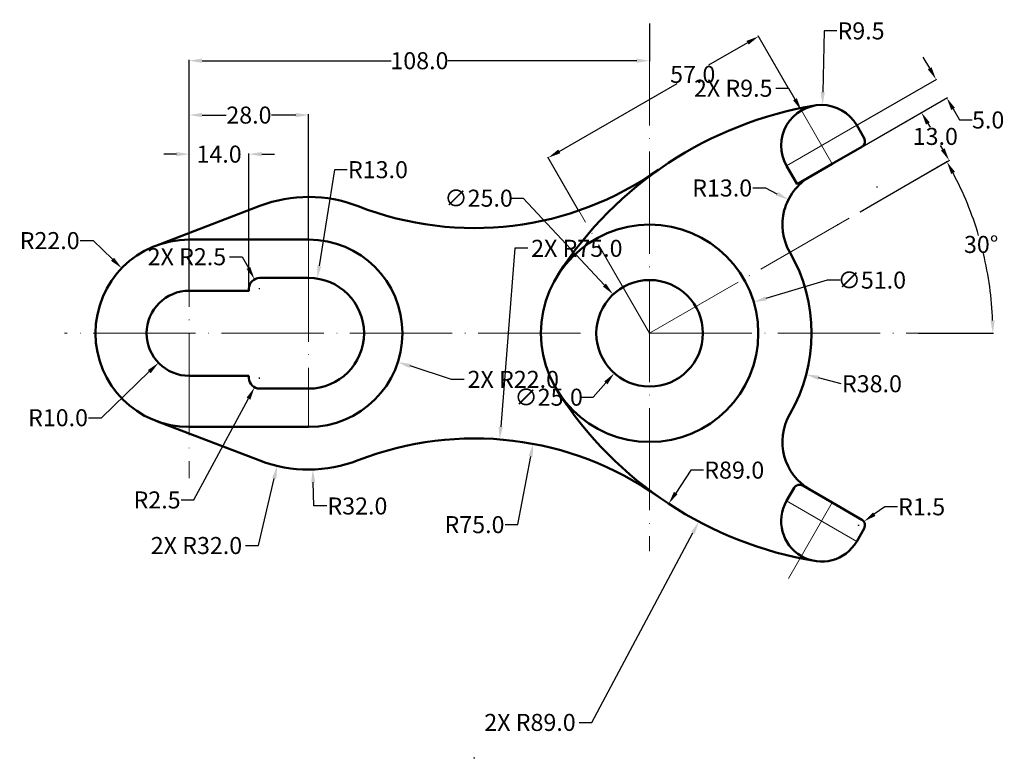
# Model space of a CAD drawing. Units: inches. Extents: x 213 to 444, y 97 to 271.
import ezdxf

# ---------------------------------------------------------------- set-up
doc = ezdxf.new("R2010")
doc.units = ezdxf.units.IN
doc.header["$MEASUREMENT"] = 0
doc.linetypes.add('ACAD_ISO04W100', pattern=[30, 24, -3, 0, -3])
for name, color, linetype, lineweight in [('M-CNTR', 4, 'ACAD_ISO04W100', 18), ('M-DIMS', 7, 'Continuous', 25), ('M-OUTL', 7, 'Continuous', 50)]:
    doc.layers.add(name, color=color, linetype=linetype, lineweight=lineweight)
doc.styles.get("Standard").update_dxf_attribs({"font": 'arial.ttf'})
doc.dimstyles.get("Standard").update_dxf_attribs({"dimtxt": 4, "dimasz": 3, "dimexe": 0.18, "dimexo": 0.0625, "dimgap": 0.09, "dimtad": 0, "dimtih": 1, "dimtoh": 1, "dimdec": 1, "dimzin": 0, "dimdsep": 46, "dimtxsty": 'Standard', "dimcen": 0.09, "dimclrd": 1, "dimclre": 1, "dimadec": 0, "dimazin": 0, "dimtfac": 1, "dimtdec": 1, "dimtofl": 0, "dimtmove": 0, "dimatfit": 3, "dimfxl": 1, "dimtolj": 1, "dimtzin": 0, "dimarcsym": 0})

# ---------------------------------------------------------------- blocks, each defined once
blk = doc.blocks.new('*D1')
at = {"layer": 'Defpoints', "color": 0, "transparency": 16777216}
for p in [(409.73, 225.61), (439.68, 211.1), (360.37, 197.11), (360.37, 197.11), (423.38, 197.11)]:
    blk.add_point(p, dxfattribs=at)
at = {"layer": 'M-DIMS', "color": 0, "lineweight": -2, "transparency": 16777216}
for p, q in [((409.78, 225.64), (430.27, 237.47)), ((423.45, 197.11), (441.08, 197.11))]:
    blk.add_line(p, q, dxfattribs=at)
for start, end in [(16.5776, 27.8655), (2.1345, 13.434)]:
    blk.add_arc((360.37, 197.11), 80.53, start, end, dxfattribs=at)
at = {"layer": 'M-DIMS', "color": 0, "transparency": 16777216}
for points in [[(431.12, 234.51), (432, 235), (430.11, 237.38)], [(441.34, 200.12), (440.34, 200.1), (440.9, 197.11)]]:
    blk.add_solid(points, dxfattribs=at)
at = {"layer": 'M-DIMS', "color": 0, "transparency": 16777216, "insert": (438.16, 217.96), "char_height": 4, "attachment_point": 5}
blk.add_mtext('\\A1;30°', dxfattribs=at)
blk = doc.blocks.new('*D2')
at = {"layer": 'Defpoints', "color": 0, "transparency": 16777216}
for p in [(360.37, 197.11), (397.11, 187.43)]:
    blk.add_point(p, dxfattribs=at)
at = {"layer": 'M-DIMS', "color": 0, "lineweight": -2, "transparency": 16777216}
for p, q in [((360.28, 197.11), (360.46, 197.11)), ((360.37, 197.02), (360.37, 197.2)), ((405.35, 185.26), (400.01, 186.66))]:
    blk.add_line(p, q, dxfattribs=at)
at = {"layer": 'M-DIMS', "color": 0, "transparency": 16777216}
blk.add_solid([(400.14, 187.15), (399.88, 186.18), (397.11, 187.43)], dxfattribs=at)
at = {"layer": 'M-DIMS', "color": 0, "transparency": 16777216, "insert": (412.54, 185.26), "char_height": 4, "attachment_point": 5}
blk.add_mtext('\\A1;R38.0', dxfattribs=at)
blk = doc.blocks.new('*D3')
at = {"layer": 'Defpoints', "color": 0, "transparency": 16777216}
for p in [(413.78, 231.45), (364.85, 157.11)]:
    blk.add_point(p, dxfattribs=at)
at = {"layer": 'M-DIMS', "color": 0, "lineweight": -2, "transparency": 16777216}
for p, q in [((370.03, 164.99), (366.5, 159.61)), ((373.03, 164.99), (370.03, 164.99))]:
    blk.add_line(p, q, dxfattribs=at)
at = {"layer": 'M-DIMS', "color": 0, "transparency": 16777216}
blk.add_solid([(366.08, 159.89), (366.91, 159.34), (364.85, 157.11)], dxfattribs=at)
at = {"layer": 'M-DIMS', "color": 0, "transparency": 16777216, "insert": (380.23, 164.99), "char_height": 4, "attachment_point": 5}
blk.add_mtext('\\A1;R89.0', dxfattribs=at)
blk = doc.blocks.new('*D4')
at = {"layer": 'Defpoints', "color": 0, "transparency": 16777216}
for p in [(400.94, 250.7), (400.73, 241.2)]:
    blk.add_point(p, dxfattribs=at)
at = {"layer": 'M-DIMS', "color": 0, "lineweight": -2, "transparency": 16777216}
for p, q in [((401.32, 268.09), (401, 253.7)), ((404.32, 268.09), (401.32, 268.09)), ((400.64, 241.2), (400.82, 241.2)), ((400.73, 241.11), (400.73, 241.29))]:
    blk.add_line(p, q, dxfattribs=at)
at = {"layer": 'M-DIMS', "color": 0, "transparency": 16777216}
blk.add_solid([(400.5, 253.71), (401.5, 253.69), (400.94, 250.7)], dxfattribs=at)
at = {"layer": 'M-DIMS', "color": 0, "transparency": 16777216, "insert": (409.98, 268.09), "char_height": 4, "attachment_point": 5}
blk.add_mtext('\\A1;R9.5', dxfattribs=at)
blk = doc.blocks.new('*D5')
at = {"layer": 'Defpoints', "color": 0, "transparency": 16777216}
for p in [(392.94, 228.49), (404.53, 222.61)]:
    blk.add_point(p, dxfattribs=at)
at = {"layer": 'M-DIMS', "color": 0, "lineweight": -2, "transparency": 16777216}
for p, q in [((384.59, 231.21), (387.59, 231.21)), ((387.59, 231.21), (390.26, 229.85)), ((404.44, 222.61), (404.62, 222.61)), ((404.53, 222.52), (404.53, 222.7))]:
    blk.add_line(p, q, dxfattribs=at)
at = {"layer": 'M-DIMS', "color": 0, "transparency": 16777216}
blk.add_solid([(390.49, 230.3), (390.04, 229.4), (392.94, 228.49)], dxfattribs=at)
at = {"layer": 'M-DIMS', "color": 0, "transparency": 16777216, "insert": (377.4, 231.21), "char_height": 4, "attachment_point": 5}
blk.add_mtext('\\A1;R13.0', dxfattribs=at)
blk = doc.blocks.new('*D6')
at = {"layer": 'Defpoints', "color": 0, "transparency": 16777216}
for p in [(384.8, 204.42), (335.94, 189.8)]:
    blk.add_point(p, dxfattribs=at)
at = {"layer": 'M-DIMS', "color": 0, "lineweight": -2, "transparency": 16777216}
for p, q in [((402.06, 209.59), (387.67, 205.28)), ((405.06, 209.59), (402.06, 209.59)), ((360.28, 197.11), (360.46, 197.11)), ((360.37, 197.02), (360.37, 197.2))]:
    blk.add_line(p, q, dxfattribs=at)
at = {"layer": 'M-DIMS', "color": 0, "transparency": 16777216}
blk.add_solid([(387.53, 205.76), (387.81, 204.81), (384.8, 204.42)], dxfattribs=at)
at = {"layer": 'M-DIMS', "color": 0, "transparency": 16777216, "insert": (412.51, 209.59), "char_height": 4, "attachment_point": 5}
blk.add_mtext('\\A1;∅51.0', dxfattribs=at)
blk = doc.blocks.new('*D7')
at = {"layer": 'Defpoints', "color": 0, "transparency": 16777216}
for p in [(430.08, 252.37), (408.96, 245.95), (410.16, 240.87)]:
    blk.add_point(p, dxfattribs=at)
at = {"layer": 'M-DIMS', "color": 0, "lineweight": -2, "transparency": 16777216}
for p, q in [((426.08, 259.3), (424.58, 261.9)), ((409.01, 245.98), (427.73, 256.79)), ((410.21, 240.9), (430.23, 252.46)), ((431.58, 249.77), (433.08, 247.18)), ((433.08, 247.18), (436.08, 247.18))]:
    blk.add_line(p, q, dxfattribs=at)
at = {"layer": 'M-DIMS', "color": 0, "transparency": 16777216}
for points in [[(426.51, 259.55), (425.64, 259.05), (427.58, 256.7)], [(432.01, 250.02), (431.14, 249.52), (430.08, 252.37)]]:
    blk.add_solid(points, dxfattribs=at)
at = {"layer": 'M-DIMS', "color": 0, "transparency": 16777216, "insert": (439.8, 247.18), "char_height": 4, "attachment_point": 5}
blk.add_mtext('\\A1;5.0', dxfattribs=at)
blk = doc.blocks.new('*D8')
at = {"layer": 'Defpoints', "color": 0, "transparency": 16777216}
for p in [(410.16, 240.87), (430.65, 237.69), (409.73, 225.61)]:
    blk.add_point(p, dxfattribs=at)
at = {"layer": 'M-DIMS', "color": 0, "lineweight": -2, "transparency": 16777216}
for p, q in [((410.21, 240.9), (424.3, 249.04)), ((425.65, 246.35), (426.16, 245.45)), ((429.15, 240.29), (428.63, 241.18)), ((409.78, 225.64), (430.8, 237.78))]:
    blk.add_line(p, q, dxfattribs=at)
at = {"layer": 'M-DIMS', "color": 0, "transparency": 16777216}
for points in [[(426.08, 246.6), (425.21, 246.1), (424.15, 248.95)], [(429.58, 240.54), (428.71, 240.04), (430.65, 237.69)]]:
    blk.add_solid(points, dxfattribs=at)
at = {"layer": 'M-DIMS', "color": 0, "transparency": 16777216, "insert": (427.4, 243.32), "char_height": 4, "attachment_point": 5}
blk.add_mtext('\\A1;13.0', dxfattribs=at)
blk = doc.blocks.new('*D9')
at = {"layer": 'Defpoints', "color": 0, "transparency": 16777216}
for p in [(410.63, 152.92), (409.41, 152.06)]:
    blk.add_point(p, dxfattribs=at)
at = {"layer": 'M-DIMS', "color": 0, "lineweight": -2, "transparency": 16777216}
for p, q in [((415.53, 156.38), (413.08, 154.65)), ((418.53, 156.38), (415.53, 156.38)), ((409.32, 152.06), (409.5, 152.06)), ((409.41, 151.97), (409.41, 152.15))]:
    blk.add_line(p, q, dxfattribs=at)
at = {"layer": 'M-DIMS', "color": 0, "transparency": 16777216}
blk.add_solid([(412.8, 155.06), (413.37, 154.24), (410.63, 152.92)], dxfattribs=at)
at = {"layer": 'M-DIMS', "color": 0, "transparency": 16777216, "insert": (424.19, 156.38), "char_height": 4, "attachment_point": 5}
blk.add_mtext('\\A1;R1.5', dxfattribs=at)
blk = doc.blocks.new('*D10')
at = {"layer": 'Defpoints', "color": 0, "transparency": 16777216}
for p in [(385.95, 266.81), (392.94, 254.7), (343.74, 225.91)]:
    blk.add_point(p, dxfattribs=at)
at = {"layer": 'M-DIMS', "color": 0, "lineweight": -2, "transparency": 16777216}
for p, q in [((392.91, 254.75), (385.86, 266.96)), ((383.35, 265.31), (374.19, 260.02)), ((339.18, 239.81), (366.8, 255.75)), ((343.71, 225.96), (336.49, 238.46))]:
    blk.add_line(p, q, dxfattribs=at)
at = {"layer": 'M-DIMS', "color": 0, "transparency": 16777216}
for points in [[(383.1, 265.74), (383.6, 264.87), (385.95, 266.81)], [(338.93, 240.24), (339.43, 239.37), (336.58, 238.31)]]:
    blk.add_solid(points, dxfattribs=at)
at = {"layer": 'M-DIMS', "color": 0, "transparency": 16777216, "insert": (370.49, 257.88), "char_height": 4, "attachment_point": 5}
blk.add_mtext('\\A1;57.0', dxfattribs=at)
blk = doc.blocks.new('*D11')
at = {"layer": 'Defpoints', "color": 0, "transparency": 16777216}
for p in [(360.37, 269.85), (360.37, 261.09), (252.37, 227.31)]:
    blk.add_point(p, dxfattribs=at)
at = {"layer": 'M-DIMS', "color": 0, "lineweight": -2, "transparency": 16777216}
for p, q in [((360.37, 269.79), (360.37, 260.91)), ((252.37, 227.38), (252.37, 261.27)), ((255.37, 261.09), (299.72, 261.09)), ((357.37, 261.09), (313.01, 261.09))]:
    blk.add_line(p, q, dxfattribs=at)
at = {"layer": 'M-DIMS', "color": 0, "transparency": 16777216}
for points in [[(255.37, 261.59), (255.37, 260.59), (252.37, 261.09)], [(357.37, 261.59), (357.37, 260.59), (360.37, 261.09)]]:
    blk.add_solid(points, dxfattribs=at)
at = {"layer": 'M-DIMS', "color": 0, "transparency": 16777216, "insert": (306.37, 261.09), "char_height": 4, "attachment_point": 5}
blk.add_mtext('\\A1;108.0', dxfattribs=at)
blk = doc.blocks.new('*D12')
at = {"layer": 'Defpoints', "color": 0, "transparency": 16777216}
for p in [(266.37, 239.16), (252.37, 207.11), (266.37, 207.11)]:
    blk.add_point(p, dxfattribs=at)
at = {"layer": 'M-DIMS', "color": 0, "lineweight": -2, "transparency": 16777216}
for p, q in [((249.37, 239.16), (246.37, 239.16)), ((252.37, 207.18), (252.37, 239.34)), ((266.37, 207.18), (266.37, 239.34)), ((269.37, 239.16), (272.37, 239.16))]:
    blk.add_line(p, q, dxfattribs=at)
at = {"layer": 'M-DIMS', "color": 0, "transparency": 16777216}
for points in [[(249.37, 239.66), (249.37, 238.66), (252.37, 239.16)], [(269.37, 239.66), (269.37, 238.66), (266.37, 239.16)]]:
    blk.add_solid(points, dxfattribs=at)
at = {"layer": 'M-DIMS', "color": 0, "transparency": 16777216, "insert": (259.37, 239.16), "char_height": 4, "attachment_point": 5}
blk.add_mtext('\\A1;14.0', dxfattribs=at)
blk = doc.blocks.new('*D13')
at = {"layer": 'Defpoints', "color": 0, "transparency": 16777216}
for p in [(280.37, 248.33), (280.37, 219.11), (252.37, 207.11)]:
    blk.add_point(p, dxfattribs=at)
at = {"layer": 'M-DIMS', "color": 0, "lineweight": -2, "transparency": 16777216}
for p, q in [((252.37, 207.18), (252.37, 248.51)), ((255.37, 248.33), (261.05, 248.33)), ((277.37, 248.33), (271.68, 248.33)), ((280.37, 219.18), (280.37, 248.51))]:
    blk.add_line(p, q, dxfattribs=at)
at = {"layer": 'M-DIMS', "color": 0, "transparency": 16777216}
for points in [[(255.37, 248.83), (255.37, 247.83), (252.37, 248.33)], [(277.37, 248.83), (277.37, 247.83), (280.37, 248.33)]]:
    blk.add_solid(points, dxfattribs=at)
at = {"layer": 'M-DIMS', "color": 0, "transparency": 16777216, "insert": (266.37, 248.33), "char_height": 4, "attachment_point": 5}
blk.add_mtext('\\A1;28.0', dxfattribs=at)
blk = doc.blocks.new('*D14')
at = {"layer": 'Defpoints', "color": 0, "transparency": 16777216}
for p in [(282.4, 209.95), (280.37, 197.11)]:
    blk.add_point(p, dxfattribs=at)
at = {"layer": 'M-DIMS', "color": 0, "lineweight": -2, "transparency": 16777216}
for p, q in [((286.45, 235.51), (282.87, 212.92)), ((289.45, 235.51), (286.45, 235.51)), ((280.28, 197.11), (280.46, 197.11)), ((280.37, 197.02), (280.37, 197.2))]:
    blk.add_line(p, q, dxfattribs=at)
at = {"layer": 'M-DIMS', "color": 0, "transparency": 16777216}
blk.add_solid([(282.38, 212.99), (283.36, 212.84), (282.4, 209.95)], dxfattribs=at)
at = {"layer": 'M-DIMS', "color": 0, "transparency": 16777216, "insert": (296.64, 235.51), "char_height": 4, "attachment_point": 5}
blk.add_mtext('\\A1;R13.0', dxfattribs=at)
blk = doc.blocks.new('*D15')
at = {"layer": 'Defpoints', "color": 0, "transparency": 16777216}
for p in [(280.37, 197.11), (281.36, 165.13)]:
    blk.add_point(p, dxfattribs=at)
at = {"layer": 'M-DIMS', "color": 0, "lineweight": -2, "transparency": 16777216}
for p, q in [((280.28, 197.11), (280.46, 197.11)), ((280.37, 197.02), (280.37, 197.2)), ((281.63, 156.57), (281.45, 162.13)), ((284.63, 156.57), (281.63, 156.57))]:
    blk.add_line(p, q, dxfattribs=at)
at = {"layer": 'M-DIMS', "color": 0, "transparency": 16777216}
blk.add_solid([(281.95, 162.15), (280.95, 162.11), (281.36, 165.13)], dxfattribs=at)
at = {"layer": 'M-DIMS', "color": 0, "transparency": 16777216, "insert": (291.82, 156.57), "char_height": 4, "attachment_point": 5}
blk.add_mtext('\\A1;R32.0', dxfattribs=at)
blk = doc.blocks.new('*D16')
at = {"layer": 'Defpoints', "color": 0, "transparency": 16777216}
for p in [(268.87, 186.61), (267.68, 184.41)]:
    blk.add_point(p, dxfattribs=at)
at = {"layer": 'M-DIMS', "color": 0, "lineweight": -2, "transparency": 16777216}
for p, q in [((268.78, 186.61), (268.96, 186.61)), ((268.87, 186.52), (268.87, 186.7)), ((253.48, 157.99), (266.26, 181.77)), ((250.48, 157.99), (253.48, 157.99))]:
    blk.add_line(p, q, dxfattribs=at)
at = {"layer": 'M-DIMS', "color": 0, "transparency": 16777216}
blk.add_solid([(265.82, 182), (266.7, 181.53), (267.68, 184.41)], dxfattribs=at)
at = {"layer": 'M-DIMS', "color": 0, "transparency": 16777216, "insert": (244.82, 157.99), "char_height": 4, "attachment_point": 5}
blk.add_mtext('\\A1;R2.5', dxfattribs=at)
blk = doc.blocks.new('*D17')
at = {"layer": 'Defpoints', "color": 0, "transparency": 16777216}
for p in [(252.37, 197.11), (245.16, 190.18)]:
    blk.add_point(p, dxfattribs=at)
at = {"layer": 'M-DIMS', "color": 0, "lineweight": -2, "transparency": 16777216}
for p, q in [((252.28, 197.11), (252.46, 197.11)), ((252.37, 197.02), (252.37, 197.2)), ((231.77, 177.29), (243, 188.1)), ((228.77, 177.29), (231.77, 177.29))]:
    blk.add_line(p, q, dxfattribs=at)
at = {"layer": 'M-DIMS', "color": 0, "transparency": 16777216}
blk.add_solid([(242.65, 188.46), (243.35, 187.74), (245.16, 190.18)], dxfattribs=at)
at = {"layer": 'M-DIMS', "color": 0, "transparency": 16777216, "insert": (221.58, 177.29), "char_height": 4, "attachment_point": 5}
blk.add_mtext('\\A1;R10.0', dxfattribs=at)
blk = doc.blocks.new('*D18')
at = {"layer": 'Defpoints', "color": 0, "transparency": 16777216}
for p in [(236.53, 212.39), (252.37, 197.11)]:
    blk.add_point(p, dxfattribs=at)
at = {"layer": 'M-DIMS', "color": 0, "lineweight": -2, "transparency": 16777216}
for p, q in [((226.81, 218.86), (229.81, 218.86)), ((229.81, 218.86), (234.37, 214.47)), ((252.28, 197.11), (252.46, 197.11)), ((252.37, 197.02), (252.37, 197.2))]:
    blk.add_line(p, q, dxfattribs=at)
at = {"layer": 'M-DIMS', "color": 0, "transparency": 16777216}
blk.add_solid([(234.72, 214.83), (234.02, 214.11), (236.53, 212.39)], dxfattribs=at)
at = {"layer": 'M-DIMS', "color": 0, "transparency": 16777216, "insert": (219.62, 218.86), "char_height": 4, "attachment_point": 5}
blk.add_mtext('\\A1;R22.0', dxfattribs=at)
blk = doc.blocks.new('*D19')
at = {"layer": 'Defpoints', "color": 0, "transparency": 16777216}
for p in [(333.02, 171.16), (319.25, 97.43)]:
    blk.add_point(p, dxfattribs=at)
at = {"layer": 'M-DIMS', "color": 0, "lineweight": -2, "transparency": 16777216}
for p, q in [((329.48, 152.19), (332.47, 168.21)), ((326.48, 152.19), (329.48, 152.19))]:
    blk.add_line(p, q, dxfattribs=at)
at = {"layer": 'M-DIMS', "color": 0, "transparency": 16777216}
blk.add_solid([(331.98, 168.3), (332.96, 168.11), (333.02, 171.16)], dxfattribs=at)
at = {"layer": 'M-DIMS', "color": 0, "transparency": 16777216, "insert": (319.29, 152.19), "char_height": 4, "attachment_point": 5}
blk.add_mtext('\\A1;R75.0', dxfattribs=at)
blk = doc.blocks.new('*D20')
at = {"layer": 'Defpoints', "color": 0, "transparency": 16777216}
for p in [(351.83, 206.24), (368.91, 187.98)]:
    blk.add_point(p, dxfattribs=at)
at = {"layer": 'M-DIMS', "color": 0, "lineweight": -2, "transparency": 16777216}
for p, q in [((327.71, 228.82), (330.71, 228.82)), ((330.71, 228.82), (349.78, 208.43)), ((360.28, 197.11), (360.46, 197.11)), ((360.37, 197.02), (360.37, 197.2))]:
    blk.add_line(p, q, dxfattribs=at)
at = {"layer": 'M-DIMS', "color": 0, "transparency": 16777216}
blk.add_solid([(350.14, 208.77), (349.41, 208.09), (351.83, 206.24)], dxfattribs=at)
at = {"layer": 'M-DIMS', "color": 0, "transparency": 16777216, "insert": (320.25, 228.82), "char_height": 4, "attachment_point": 5}
blk.add_mtext('\\A1;∅25.0', dxfattribs=at)
blk = doc.blocks.new('*D21')
at = {"layer": 'Defpoints', "color": 0, "transparency": 16777216}
for p in [(280.37, 197.11), (301.3, 190.35)]:
    blk.add_point(p, dxfattribs=at)
at = {"layer": 'M-DIMS', "color": 1, "lineweight": -2, "transparency": 16777216}
for p, q in [((280.28, 197.11), (280.46, 197.11)), ((280.37, 197.02), (280.37, 197.2)), ((313.86, 186.29), (304.16, 189.43)), ((316.86, 186.29), (313.86, 186.29))]:
    blk.add_line(p, q, dxfattribs=at)
at = {"layer": 'M-DIMS', "color": 1, "transparency": 16777216}
blk.add_solid([(304.31, 189.9), (304, 188.95), (301.3, 190.35)], dxfattribs=at)
at = {"layer": 'M-DIMS', "color": 0, "transparency": 16777216, "insert": (328.39, 186.29), "char_height": 4, "attachment_point": 5}
blk.add_mtext('\\A1;2X R22.0', dxfattribs=at)
blk = doc.blocks.new('*D22')
at = {"layer": 'Defpoints', "color": 0, "transparency": 16777216}
for p in [(280.37, 197.11), (273, 165.97)]:
    blk.add_point(p, dxfattribs=at)
at = {"layer": 'M-DIMS', "color": 1, "lineweight": -2, "transparency": 16777216}
for p, q in [((280.28, 197.11), (280.46, 197.11)), ((280.37, 197.02), (280.37, 197.2)), ((268.58, 147.29), (272.31, 163.05)), ((265.58, 147.29), (268.58, 147.29))]:
    blk.add_line(p, q, dxfattribs=at)
at = {"layer": 'M-DIMS', "color": 1, "transparency": 16777216}
blk.add_solid([(271.82, 163.17), (272.8, 162.94), (273, 165.97)], dxfattribs=at)
at = {"layer": 'M-DIMS', "color": 0, "transparency": 16777216, "insert": (254.06, 147.29), "char_height": 4, "attachment_point": 5}
blk.add_mtext('\\A1;2X R32.0', dxfattribs=at)
blk = doc.blocks.new('*D23')
at = {"layer": 'Defpoints', "color": 0, "transparency": 16777216}
for p in [(267.67, 209.81), (268.87, 207.61)]:
    blk.add_point(p, dxfattribs=at)
at = {"layer": 'M-DIMS', "color": 1, "lineweight": -2, "transparency": 16777216}
for p, q in [((261.81, 215.08), (264.81, 215.08)), ((264.81, 215.08), (266.24, 212.45)), ((268.78, 207.61), (268.96, 207.61)), ((268.87, 207.52), (268.87, 207.7))]:
    blk.add_line(p, q, dxfattribs=at)
at = {"layer": 'M-DIMS', "color": 1, "transparency": 16777216}
blk.add_solid([(266.68, 212.68), (265.8, 212.21), (267.67, 209.81)], dxfattribs=at)
at = {"layer": 'M-DIMS', "color": 0, "transparency": 16777216, "insert": (251.82, 215.08), "char_height": 4, "attachment_point": 5}
blk.add_mtext('\\A1;2X R2.5', dxfattribs=at)
blk = doc.blocks.new('*D24')
at = {"layer": 'Defpoints', "color": 0, "transparency": 16777216}
for p in [(325.21, 172.19), (319.25, 97.43)]:
    blk.add_point(p, dxfattribs=at)
at = {"layer": 'M-DIMS', "color": 1, "lineweight": -2, "transparency": 16777216}
for p, q in [((328.78, 217.05), (325.45, 175.18)), ((331.78, 217.05), (328.78, 217.05)), ((319.16, 97.43), (319.34, 97.43)), ((319.25, 97.34), (319.25, 97.52))]:
    blk.add_line(p, q, dxfattribs=at)
at = {"layer": 'M-DIMS', "color": 1, "transparency": 16777216}
blk.add_solid([(324.95, 175.22), (325.94, 175.14), (325.21, 172.19)], dxfattribs=at)
at = {"layer": 'M-DIMS', "color": 0, "transparency": 16777216, "insert": (343.3, 217.05), "char_height": 4, "attachment_point": 5}
blk.add_mtext('\\A1;2X R75.0', dxfattribs=at)
blk = doc.blocks.new('*D25')
at = {"layer": 'Defpoints', "color": 0, "transparency": 16777216}
for p in [(368.63, 206.49), (352.1, 187.73)]:
    blk.add_point(p, dxfattribs=at)
at = {"layer": 'M-DIMS', "color": 1, "lineweight": -2, "transparency": 16777216}
for p, q in [((360.28, 197.11), (360.46, 197.11)), ((360.37, 197.02), (360.37, 197.2)), ((347.15, 182.11), (350.12, 185.48)), ((344.15, 182.11), (347.15, 182.11))]:
    blk.add_line(p, q, dxfattribs=at)
at = {"layer": 'M-DIMS', "color": 1, "transparency": 16777216}
blk.add_solid([(349.74, 185.81), (350.5, 185.15), (352.1, 187.73)], dxfattribs=at)
at = {"layer": 'M-DIMS', "color": 0, "transparency": 16777216, "insert": (336.69, 182.11), "char_height": 4, "attachment_point": 5}
blk.add_mtext('\\A1;∅25.0', dxfattribs=at)
blk = doc.blocks.new('*D26')
at = {"layer": 'Defpoints', "color": 0, "transparency": 16777216}
for p in [(413.78, 231.45), (371.94, 152.9)]:
    blk.add_point(p, dxfattribs=at)
at = {"layer": 'M-DIMS', "color": 1, "lineweight": -2, "transparency": 16777216}
for p, q in [((413.69, 231.45), (413.87, 231.45)), ((413.78, 231.36), (413.78, 231.54)), ((346.83, 105.77), (370.53, 150.25)), ((343.83, 105.77), (346.83, 105.77))]:
    blk.add_line(p, q, dxfattribs=at)
at = {"layer": 'M-DIMS', "color": 1, "transparency": 16777216}
blk.add_solid([(370.09, 150.48), (370.97, 150.01), (371.94, 152.9)], dxfattribs=at)
at = {"layer": 'M-DIMS', "color": 0, "transparency": 16777216, "insert": (332.31, 105.77), "char_height": 4, "attachment_point": 5}
blk.add_mtext('\\A1;2X R89.0', dxfattribs=at)
blk = doc.blocks.new('*D27')
at = {"layer": 'Defpoints', "color": 0, "transparency": 16777216}
for p in [(395.98, 249.43), (400.73, 241.2)]:
    blk.add_point(p, dxfattribs=at)
at = {"layer": 'M-DIMS', "color": 1, "lineweight": -2, "transparency": 16777216}
for p, q in [((389.98, 254.63), (392.98, 254.63)), ((392.98, 254.63), (394.48, 252.03)), ((400.64, 241.2), (400.82, 241.2)), ((400.73, 241.11), (400.73, 241.29))]:
    blk.add_line(p, q, dxfattribs=at)
at = {"layer": 'M-DIMS', "color": 1, "transparency": 16777216}
blk.add_solid([(394.91, 252.28), (394.05, 251.78), (395.98, 249.43)], dxfattribs=at)
at = {"layer": 'M-DIMS', "color": 0, "transparency": 16777216, "insert": (379.99, 254.63), "char_height": 4, "attachment_point": 5}
blk.add_mtext('\\A1;2X R9.5', dxfattribs=at)

msp = doc.modelspace()

# ---------------------------------------------------------------- linework, layer by layer
at = {"layer": 'M-CNTR'}
for p, q in [((360.37, 269.85), (360.37, 145.94)), ((403.23, 236.87), (392.94, 254.7)), ((392.5, 236.45), (408.96, 245.95)), ((252.37, 227.31), (252.37, 163.07)), ((360.37, 197.11), (343.74, 225.91)), ((360.37, 197.11), (409.73, 225.61)), ((280.37, 219.11), (280.37, 175.11)), ((344.16, 197.11), (223.13, 197.11)), ((360.37, 197.11), (423.38, 197.11)), ((392.5, 157.77), (408.96, 148.27)), ((403.23, 157.35), (392.94, 139.53))]:
    msp.add_line(p, q, dxfattribs=at)
at = {"layer": 'M-OUTL'}
for p, q in [((410.71, 242.92), (408.96, 245.95)), ((403.23, 236.87), (410.16, 240.87)), ((395, 232.12), (392.5, 236.45)), ((395, 232.12), (403.23, 236.87)), ((244.51, 217.66), (268.94, 227)), ((244.51, 176.56), (268.94, 167.22)), ((394.25, 160.81), (392.5, 157.77)), ((396.3, 161.35), (403.23, 157.35)), ((403.23, 157.35), (410.16, 153.35)), ((410.71, 151.31), (408.96, 148.27))]:
    msp.add_line(p, q, dxfattribs=at)
for points in [[(252.37, 175.11), (266.37, 175.11), (280.37, 175.11, 1), (280.37, 219.11), (266.37, 219.11), (252.37, 219.11, 1)], [(266.37, 187.11), (252.37, 187.11, -1), (252.37, 207.11), (266.37, 207.11), (266.37, 207.61, -0.414214), (268.87, 210.11), (280.37, 210.11, -1), (280.37, 184.11), (268.87, 184.11, -0.414214), (266.37, 186.61)]]:
    msp.add_lwpolyline(points, format="xyb", close=True, dxfattribs=at)
for radius in [25.5, 12.5]:
    msp.add_circle((360.37, 197.11), radius, dxfattribs=at)
for centre, radius, start, end in [((413.78, 162.78), 89, 99.4517, 147.271), ((400.73, 241.2), 9.5, 30, 210), ((409.41, 242.17), 1.5, 300, 30), ((319.25, 296.8), 75, 248.6881, 305.1979), ((404.53, 222.61), 13, 120, 210), ((280.37, 197.11), 32, 68.6881, 110.9248), ((360.37, 197.11), 38, 330, 30), ((413.78, 231.45), 89, 212.729, 260.5483), ((404.53, 171.61), 13, 150, 240), ((319.25, 97.43), 75, 54.8021, 111.3119), ((280.37, 197.11), 32, 249.0752, 291.3119), ((395.55, 160.06), 1.5, 60, 150), ((400.73, 153.02), 9.5, 150, 330), ((409.41, 152.06), 1.5, 330, 60)]:
    msp.add_arc(centre, radius, start, end, dxfattribs=at)

# ---------------------------------------------------------------- dimensions: what is measured, and where the dimension line sits
at = {"layer": 'M-DIMS'}
for center, mpoint, picture, middle in [((400.73, 241.2), (400.94, 250.7), '*D4', (409.98, 268.09)), ((280.37, 197.11), (282.4, 209.95), '*D14', (296.64, 235.51)), ((413.78, 231.45), (364.85, 157.11), '*D3', (380.23, 164.99)), ((252.37, 197.11), (236.53, 212.39), '*D18', (219.62, 218.86)), ((252.37, 197.11), (245.16, 190.18), '*D17', (221.58, 177.29)), ((280.37, 197.11), (281.36, 165.13), '*D15', (291.82, 156.57)), ((360.37, 197.11), (397.11, 187.43), '*D2', (405.35, 185.26)), ((268.87, 186.61), (267.68, 184.41), '*D16', (244.82, 157.99)), ((319.25, 97.43), (333.02, 171.16), '*D19', (319.29, 152.19))]:
    dim = msp.add_radius_dim(center=center, mpoint=mpoint, dimstyle='Standard', override={"dimclrd": 0, "dimclre": 0, "dimclrt": 0}, dxfattribs=at)
    dim.commit()
    dim.dimension.update_dxf_attribs({"geometry": picture, "text_midpoint": middle, "dimtype": 164})
for base, p1, p2, picture, middle in [((360.37, 261.09), (252.37, 227.31), (360.37, 269.85), '*D11', (306.37, 261.09)), ((280.37, 248.33), (252.37, 207.11), (280.37, 219.11), '*D13', (266.37, 248.33)), ((266.37, 239.16), (252.37, 207.11), (266.37, 207.11), '*D12', (259.37, 239.16))]:
    dim = msp.add_linear_dim(base=base, p1=p1, p2=p2, dimstyle='Standard', override={"dimclrd": 0, "dimclre": 0, "dimclrt": 0}, dxfattribs=at)
    dim.commit()
    dim.dimension.update_dxf_attribs({"geometry": picture, "text_midpoint": middle})
dim = msp.add_linear_dim(base=(385.95, 266.81), p1=(343.74, 225.91), p2=(392.94, 254.7), angle=210, dimstyle='Standard', override={"dimclrd": 0, "dimclre": 0, "dimclrt": 0}, dxfattribs=at)
dim.commit()
dim.dimension.update_dxf_attribs({"geometry": '*D10', "text_midpoint": (370.49, 257.88), "dimtype": 160})
for base, p1, p2, picture, middle in [((430.08, 252.37), (408.96, 245.95), (410.16, 240.87), '*D7', (439.8, 247.18)), ((430.65, 237.69), (410.16, 240.87), (409.73, 225.61), '*D8', (427.4, 243.32))]:
    dim = msp.add_linear_dim(base=base, p1=p1, p2=p2, angle=120, dimstyle='Standard', override={"dimclrd": 0, "dimclre": 0, "dimclrt": 0}, dxfattribs=at)
    dim.commit()
    dim.dimension.update_dxf_attribs({"geometry": picture, "text_midpoint": middle})
for center, mpoint, picture, middle in [((400.73, 241.2), (395.98, 249.43), '*D27', (379.99, 254.63)), ((268.87, 207.61), (267.67, 209.81), '*D23', (251.82, 215.08))]:
    dim = msp.add_radius_dim(center=center, mpoint=mpoint, text='2X <>', dimstyle='Standard', override={"dimdec": 1, "dimlfac": 1, "dimrnd": 0, "dimzin": 0, "dimdsep": 46, "dimlunit": 2}, dxfattribs=at)
    dim.commit()
    dim.dimension.update_dxf_attribs({"geometry": picture, "text_midpoint": middle})
dim = msp.add_angular_dim_2l(base=(439.68, 211.1), line1=((360.37, 197.11), (423.38, 197.11)), line2=((360.37, 197.11), (409.73, 225.61)), dimstyle='Standard', override={"dimclrd": 0, "dimclre": 0, "dimclrt": 0}, dxfattribs=at)
dim.commit()
dim.dimension.update_dxf_attribs({"geometry": '*D1', "text_midpoint": (438.16, 217.96)})
for center, mpoint, picture, middle in [((404.53, 222.61), (392.94, 228.49), '*D5', (377.4, 231.21)), ((409.41, 152.06), (410.63, 152.92), '*D9', (424.19, 156.38))]:
    dim = msp.add_radius_dim(center=center, mpoint=mpoint, dimstyle='Standard', override={"dimclrd": 0, "dimclre": 0, "dimclrt": 0}, dxfattribs=at)
    dim.commit()
    dim.dimension.update_dxf_attribs({"geometry": picture, "text_midpoint": middle})
for p1, p2, override, picture, middle in [((368.91, 187.98), (351.83, 206.24), {"dimclrd": 0, "dimclre": 0, "dimclrt": 0}, '*D20', (320.25, 228.82)), ((335.94, 189.8), (384.8, 204.42), {"dimclrd": 0, "dimclre": 0, "dimclrt": 0}, '*D6', (412.51, 209.59)), ((368.63, 206.49), (352.1, 187.73), {"dimdec": 1, "dimlfac": 1, "dimrnd": 0, "dimzin": 0, "dimdsep": 46, "dimlunit": 2}, '*D25', (336.69, 182.11))]:
    dim = msp.add_diameter_dim_2p(p1=p1, p2=p2, dimstyle='Standard', override=override, dxfattribs=at)
    dim.commit()
    dim.dimension.update_dxf_attribs({"geometry": picture, "text_midpoint": middle, "dimtype": 163})
for center, mpoint, picture, middle in [((413.78, 231.45), (371.94, 152.9), '*D26', (332.31, 105.77)), ((319.25, 97.43), (325.21, 172.19), '*D24', (343.3, 217.05)), ((280.37, 197.11), (273, 165.97), '*D22', (254.06, 147.29)), ((280.37, 197.11), (301.3, 190.35), '*D21', (328.39, 186.29))]:
    dim = msp.add_radius_dim(center=center, mpoint=mpoint, text='2X <>', dimstyle='Standard', override={"dimdec": 1, "dimlfac": 1, "dimrnd": 0, "dimzin": 0, "dimdsep": 46, "dimlunit": 2}, dxfattribs=at)
    dim.commit()
    dim.dimension.update_dxf_attribs({"geometry": picture, "text_midpoint": middle, "dimtype": 164})

doc.saveas('drawing.dxf')
